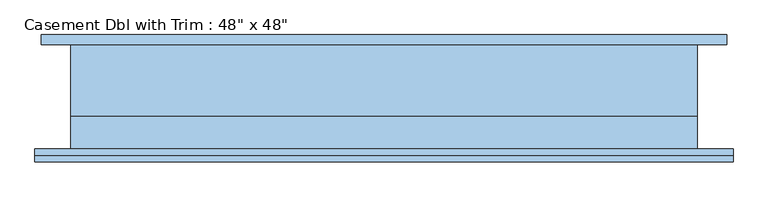
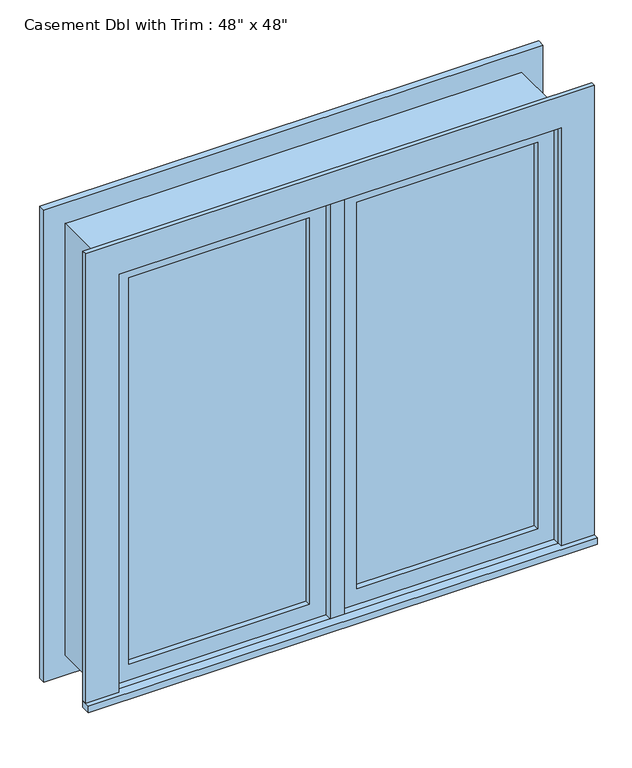
"""IFC4 building model written with IfcOpenShell, lengths in millimetres: window geometry."""

from ifc_helpers import new_model, si_unit, frame, origin, place, context, project, spatial, polyline, outline, extrude, source, transform, mapped, element, save


def window_3a1167bf(model_context):
    return source(origin(), model_context, "Body", "SweptSolid", [
        extrude(outline(polyline([(63.5, -85.725), (63.5, -73.025), (546.1, -73.025), (546.1, -85.725), (63.5, -85.725)])), frame((0.0, 0.0, 977.9), z_axis=(0.0, 0.0, 1.0), x_axis=(1.0, 0.0, 0.0)), (0.0, 0.0, 1.0), 1092.2),
        extrude(outline(polyline([(2114.55, 19.05), (933.45, 19.05), (933.45, 590.55), (2114.55, 590.55), (2114.55, 19.05)]), holes=[polyline([(2070.1, 63.5), (2070.1, 546.1), (977.9, 546.1), (977.9, 63.5), (2070.1, 63.5)])]), frame((0.0, -101.6, 0.0), z_axis=(0.0, 1.0, 0.0), x_axis=(0.0, 0.0, 1.0)), (0.0, 0.0, 1.0), 44.45),
        extrude(outline(polyline([(19.05, -57.15), (19.05, -120.65), (-19.05, -120.65), (-19.05, -57.15), (19.05, -57.15)])), frame((0.0, 0.0, 933.45), z_axis=(0.0, 0.0, 1.0), x_axis=(1.0, 0.0, 0.0)), (0.0, 0.0, 1.0), 1181.1),
        extrude(outline(polyline([(-679.45, -146.05), (-679.45, -120.65), (679.45, -120.65), (679.45, -146.05), (-679.45, -146.05)])), frame((0.0, 0.0, 914.4), z_axis=(0.0, 0.0, 1.0), x_axis=(1.0, 0.0, 0.0)), (0.0, 0.0, 1.0), 19.05),
        extrude(outline(polyline([(2114.55, -590.55), (2114.55, 590.55), (933.45, 590.55), (933.45, 679.45), (2203.45, 679.45), (2203.45, -679.45), (933.45, -679.45), (933.45, -590.55), (2114.55, -590.55)])), frame((0.0, -133.35, 0.0), z_axis=(0.0, 1.0, 0.0), x_axis=(0.0, 0.0, 1.0)), (0.0, 0.0, 1.0), 12.7),
        extrude(outline(polyline([(2190.75, 666.75), (2190.75, -666.75), (857.25, -666.75), (857.25, 666.75), (2190.75, 666.75)]), holes=[polyline([(2101.85, 577.85), (946.15, 577.85), (946.15, -577.85), (2101.85, -577.85), (2101.85, 577.85)])]), frame((0.0, 82.55, 0.0), z_axis=(0.0, 1.0, 0.0), x_axis=(0.0, 0.0, 1.0)), (0.0, 0.0, 1.0), 19.05),
        extrude(outline(polyline([(-63.5, -73.025), (-63.5, -85.725), (-546.1, -85.725), (-546.1, -73.025), (-63.5, -73.025)])), frame((0.0, 0.0, 977.9), z_axis=(0.0, 0.0, 1.0), x_axis=(1.0, 0.0, 0.0)), (0.0, 0.0, 1.0), 1092.2),
        extrude(outline(polyline([(2114.55, -590.55), (933.45, -590.55), (933.45, -19.05), (2114.55, -19.05), (2114.55, -590.55)]), holes=[polyline([(2070.1, -546.1), (2070.1, -63.5), (977.9, -63.5), (977.9, -546.1), (2070.1, -546.1)])]), frame((0.0, -101.6, 0.0), z_axis=(0.0, 1.0, 0.0), x_axis=(0.0, 0.0, 1.0)), (0.0, 0.0, 1.0), 44.45),
        extrude(outline(polyline([(2133.6, -609.6), (914.4, -609.6), (914.4, 609.6), (2133.6, 609.6), (2133.6, -609.6)]), holes=[polyline([(2101.85, -577.85), (2101.85, 577.85), (946.15, 577.85), (946.15, -577.85), (2101.85, -577.85)])]), frame((0.0, -57.15, 0.0), z_axis=(0.0, 1.0, 0.0), x_axis=(0.0, 0.0, 1.0)), (0.0, 0.0, 1.0), 139.7),
        extrude(outline(polyline([(2133.6, 609.6), (2133.6, -609.6), (914.4, -609.6), (914.4, 609.6), (2133.6, 609.6)]), holes=[polyline([(2114.55, 590.55), (933.45, 590.55), (933.45, -590.55), (2114.55, -590.55), (2114.55, 590.55)])]), frame((0.0, -120.65, 0.0), z_axis=(0.0, 1.0, 0.0), x_axis=(0.0, 0.0, 1.0)), (0.0, 0.0, 1.0), 63.5),
    ])


if __name__ == "__main__":
    model = new_model("IFC4")
    model_context = context("Model", 3, world=origin())
    ifc_project = project(units=[si_unit("LENGTHUNIT", "METRE", prefix="MILLI")], contexts=[model_context])
    site = spatial("IfcSite", under=ifc_project)
    building = spatial("IfcBuilding", under=site)
    placement = place(None, origin())
    window_shape = window_3a1167bf(model_context)
    element("IfcWindow", 1, ObjectType="Casement Dbl with Trim : 48\" x 48\"", at=placement, inside=building, context=model_context, shape_type="MappedRepresentation", body=[
        mapped(window_shape, transform((0.0, 0.0, 0.0), x_axis=(1.0, 0.0, 0.0), y_axis=(0.0, 1.0, 0.0), z_axis=(0.0, 0.0, 1.0))),
    ])
    save(model, "model.ifc")

# Revit data of these elements
# Type "Casement Dbl with Trim : 48\" x 48\""
#   Type Mark = "10"
#   Construction Type Id = "GSP4R"
#   Assembly Code = "B2020100"
#   Analytic Construction = "1/8 in Pilkington single glazing"
#   Visual Light Transmittance = 0.9
#   Solar Heat Gain Coefficient = 0.78
#   Heat Transfer Coefficient (U) = 0.6496 BTU/(h·ft²·°F)
#   Height = 4' - 0"
#   Default Sill Height = 3' - 0"
#   Trim Projection - Ext. = 0' - 0 1/2"
#   Trim Projection - Int. = 0' - 0 3/4"
#   Trim Width - Exterior = 0' - 3 1/2"
#   Trim Width - Interior = 0' - 3 1/2"
#   Width = 4' - 0"
#   Window Inset = 0' - 0 3/4"
#   Define Thermal Properties by = 1
#   Glass Pane Material = Glass
#   Sash Material = Sash
#   Trim Exterior Material = Trim
#   Trim Interior Material = Trim
#   Wall Closure = (empty or 0)
# Element 1 (IfcWindow, "Casement Dbl with Trim : 48\" x 48\"")
#   Materials on its faces: "Sash", "Trim", "Glass"
# Materials
#   "Glass": class "Glass", colour RGB 0 128 192, transparency 0.75, Description = "Soda Lime Glass", Cost = 0
#   "Sash": class "Wood", colour RGB 224 178 126, transparency 0
#   "Trim": class "Wood", colour RGB 224 178 126, transparency 0
